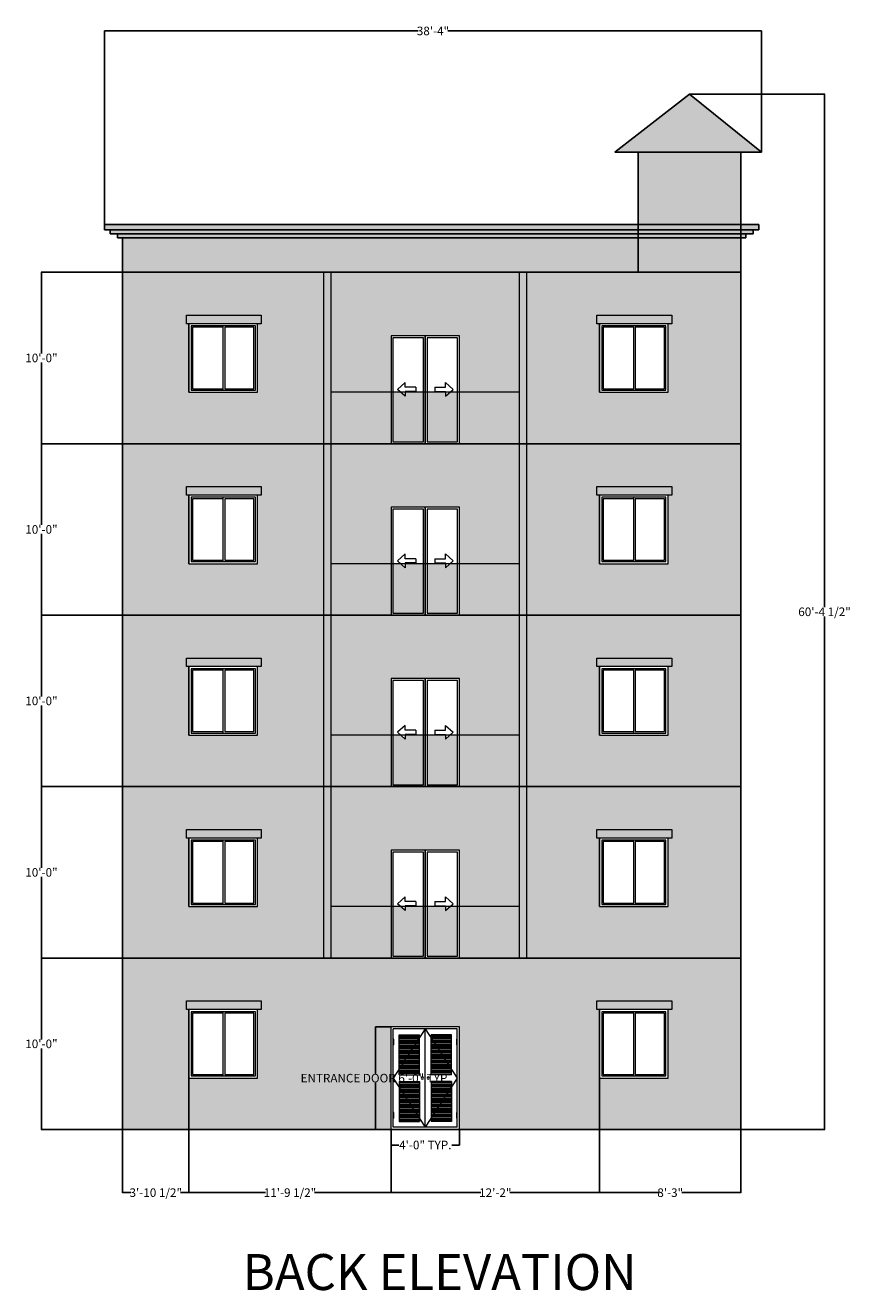
# Model space of a CAD drawing. Units: inches. Extents: x -113 to 5399, y -1393 to 3302.
# Tile 22 of 40: x 4822 to 5399, y -1393 to -507. Entities that reach past the tile are written whole.
import ezdxf

# ---------------------------------------------------------------- set-up
doc = ezdxf.new("R2010")
doc.units = ezdxf.units.IN
doc.header["$MEASUREMENT"] = 0
for name, color, linetype, lineweight in [('A-ANNO-DIMS', 254, 'Continuous', 18), ('A-ANNO-TEXT', 7, 'Continuous', 25), ('A-Door', 150, 'Continuous', 18), ('A-ELEV', 7, 'Continuous', 25), ('A-ELEV-GLAZ', 150, 'Continuous', 18), ('A-ELEV-RAIL', 7, 'Continuous', 18), ('A-ELEV-TRIM', 7, 'Continuous', 18), ('A-ELEV-TRIM-PATT', 7, 'Continuous', 13), ('A-ROOF', 7, 'Continuous', 25), ('A-ROOF-CORN-PATT', 3, 'Continuous', 13)]:
    doc.layers.add(name, color=color, linetype=linetype, lineweight=lineweight)
for name, color, linetype, lineweight, true_color in [('A-ELEV-RAIL-PATT', 9, 'Continuous', 13, 0xc7c8ca), ('A-ELEV-WALL-PATT', 241, 'Continuous', 13, 0xf7abae), ('A-ROOF-PATT', 251, 'Continuous', 13, 0x636466)]:
    doc.layers.add(name, color=color, linetype=linetype, lineweight=lineweight, true_color=true_color)
doc.styles.get("Standard").update_dxf_attribs({"font": 'arial.ttf'})
doc.dimstyles.get("Standard").update_dxf_attribs({"dimtxt": 6, "dimasz": 0.18, "dimexe": 0.18, "dimexo": 0.0625, "dimgap": 0.09, "dimtad": 0, "dimtih": 1, "dimtoh": 1, "dimdec": 1, "dimzin": 0, "dimdsep": 46, "dimlunit": 4, "dimtxsty": 'Standard', "dimblk": 'ARCHTICK', "dimcen": 0.09, "dimadec": 0, "dimazin": 0, "dimtfac": 1, "dimtdec": 1, "dimtofl": 0, "dimtmove": 0, "dimatfit": 3, "dimfxl": 1, "dimtolj": 1, "dimtzin": 0, "dimarcsym": 0})

# ---------------------------------------------------------------- blocks, each defined once
blk = doc.blocks.new('AE0C11')
for p, q in [((0, 0), (0, 1800)), ((0, 1800), (1200, 1800)), ((1200, 0), (1200, 1800)), ((40, 40), (40, 1760)), ((40, 1760), (1160, 1760)), ((600, 1760), (40, 900)), ((40, 1580), (50, 1580)), ((50, 1480), (50, 1580)), ((140, 1660), (500, 1660)), ((140, 960), (140, 1660)), ((140, 1635), (500, 1635)), ((140, 1610), (500, 1610)), ((140, 1585), (500, 1585)), ((140, 1560), (500, 1560)), ((500, 960), (500, 1660)), ((600, 40), (600, 1760)), ((600, 1760), (1160, 900)), ((700, 960), (700, 1660)), ((1060, 1660), (700, 1660)), ((1060, 1635), (700, 1635)), ((1060, 1610), (700, 1610)), ((1060, 1585), (700, 1585)), ((1060, 1560), (700, 1560)), ((1060, 960), (1060, 1660)), ((1150, 1480), (1150, 1580)), ((1150, 1580), (1160, 1580)), ((1160, 40), (1160, 1760)), ((40, 1480), (50, 1480)), ((140, 1535), (500, 1535)), ((140, 1510), (500, 1510)), ((140, 1485), (500, 1485)), ((140, 1460), (500, 1460)), ((140, 1435), (500, 1435)), ((140, 1410), (500, 1410)), ((140, 1385), (500, 1385)), ((140, 1360), (500, 1360)), ((140, 1335), (500, 1335)), ((1060, 1535), (700, 1535)), ((1060, 1510), (700, 1510)), ((1060, 1485), (700, 1485)), ((1060, 1460), (700, 1460)), ((1060, 1435), (700, 1435)), ((1060, 1410), (700, 1410)), ((1060, 1385), (700, 1385)), ((1060, 1360), (700, 1360)), ((1060, 1335), (700, 1335)), ((1150, 1480), (1160, 1480)), ((140, 1310), (500, 1310)), ((140, 1285), (500, 1285)), ((140, 1260), (500, 1260)), ((140, 1235), (500, 1235)), ((140, 1210), (500, 1210)), ((140, 1185), (500, 1185)), ((140, 1160), (500, 1160)), ((140, 1135), (500, 1135)), ((140, 1110), (500, 1110)), ((1060, 1310), (700, 1310)), ((1060, 1285), (700, 1285)), ((1060, 1260), (700, 1260)), ((1060, 1235), (700, 1235)), ((1060, 1210), (700, 1210)), ((1060, 1185), (700, 1185)), ((1060, 1160), (700, 1160)), ((1060, 1135), (700, 1135)), ((1060, 1110), (700, 1110)), ((40, 900), (600, 40)), ((140, 1085), (500, 1085)), ((140, 1060), (500, 1060)), ((140, 1035), (500, 1035)), ((140, 1010), (500, 1010)), ((140, 985), (500, 985)), ((140, 960), (500, 960)), ((1160, 900), (600, 40)), ((1060, 1085), (700, 1085)), ((1060, 1060), (700, 1060)), ((1060, 1035), (700, 1035)), ((1060, 1010), (700, 1010)), ((1060, 985), (700, 985)), ((1060, 960), (700, 960)), ((140, 840), (500, 840)), ((140, 840), (140, 140)), ((140, 815), (500, 815)), ((140, 790), (500, 790)), ((140, 765), (500, 765)), ((140, 740), (500, 740)), ((140, 715), (500, 715)), ((140, 690), (500, 690)), ((140, 665), (500, 665)), ((500, 840), (500, 140)), ((700, 840), (700, 140)), ((1060, 840), (700, 840)), ((1060, 815), (700, 815)), ((1060, 790), (700, 790)), ((1060, 765), (700, 765)), ((1060, 740), (700, 740)), ((1060, 715), (700, 715)), ((1060, 690), (700, 690)), ((1060, 665), (700, 665)), ((1060, 840), (1060, 140)), ((140, 640), (500, 640)), ((140, 615), (500, 615)), ((140, 590), (500, 590)), ((140, 565), (500, 565)), ((140, 540), (500, 540)), ((140, 515), (500, 515)), ((140, 490), (500, 490)), ((140, 465), (500, 465)), ((1060, 640), (700, 640)), ((1060, 615), (700, 615)), ((1060, 590), (700, 590)), ((1060, 565), (700, 565)), ((1060, 540), (700, 540)), ((1060, 515), (700, 515)), ((1060, 490), (700, 490)), ((1060, 465), (700, 465)), ((50, 300), (40, 300)), ((50, 200), (50, 300)), ((140, 440), (500, 440)), ((140, 415), (500, 415)), ((140, 390), (500, 390)), ((140, 365), (500, 365)), ((140, 340), (500, 340)), ((140, 315), (500, 315)), ((140, 290), (500, 290)), ((140, 265), (500, 265)), ((140, 240), (500, 240)), ((1060, 440), (700, 440)), ((1060, 415), (700, 415)), ((1060, 390), (700, 390)), ((1060, 365), (700, 365)), ((1060, 340), (700, 340)), ((1060, 315), (700, 315)), ((1060, 290), (700, 290)), ((1060, 265), (700, 265)), ((1060, 240), (700, 240)), ((1150, 300), (1160, 300)), ((1150, 200), (1150, 300)), ((0, 0), (1200, 0)), ((50, 200), (40, 200)), ((40, 40), (1160, 40)), ((140, 215), (500, 215)), ((140, 190), (500, 190)), ((140, 165), (500, 165)), ((140, 140), (500, 140)), ((1060, 215), (700, 215)), ((1060, 190), (700, 190)), ((1060, 165), (700, 165)), ((1060, 140), (700, 140)), ((1150, 200), (1160, 200))]:
    blk.add_line(p, q)
for centre in [(550, 900), (650, 900)]:
    blk.add_circle(centre, 20)
blk = doc.blocks.new('*U84')
for p, q in [((1.5, 1.5), (1.5, 46.5)), ((1.5, 46.5), (24, 46.5)), ((24, 1.5), (24, 46.5)), ((24, 46.5), (46.5, 46.5)), ((46.5, 46.5), (46.5, 1.5)), ((24, 1.5), (1.5, 1.5)), ((46.5, 1.5), (24, 1.5))]:
    blk.add_line(p, q)
blk.add_lwpolyline([(0, 0), (0, 48), (48, 48), (48, 0)], close=True)
for points in [[(23, 45.5), (23, 2.5), (2.5, 2.5), (2.5, 45.5), (23, 45.5)], [(24, 45.5), (45.5, 45.5), (45.5, 2.5), (24, 2.5)]]:
    blk.add_lwpolyline(points)
blk = doc.blocks.new('DOOR-SLIDING-PAIR-ELEV')
for p, q in [((9.94, 42.86), (4.53, 38.04)), ((9.94, 33.21), (4.53, 38.04)), ((9.94, 39.54), (9.94, 42.86)), ((17.43, 39.54), (9.94, 39.54)), ((17.43, 36.54), (9.94, 36.54)), ((9.94, 36.54), (9.94, 33.21)), ((17.43, 39.54), (17.43, 36.54)), ((30.57, 39.54), (38.06, 39.54)), ((30.57, 39.54), (30.57, 36.54)), ((30.57, 36.54), (38.06, 36.54)), ((38.06, 39.54), (38.06, 42.86)), ((38.06, 42.86), (43.47, 38.04)), ((38.06, 33.21), (43.47, 38.04)), ((38.06, 36.54), (38.06, 33.21))]:
    blk.add_line(p, q)
for points in [[(0, 75.57), (24, 75.57), (24, 0), (0, 0)], [(1.37, 74.2), (22.63, 74.2), (22.63, 1.37), (1.37, 1.37)], [(24, 75.57), (48, 75.57), (48, 0), (24, 0)], [(25.37, 74.2), (46.63, 74.2), (46.63, 1.37), (25.37, 1.37)]]:
    blk.add_lwpolyline(points, close=True)
blk = doc.blocks.new('_ArchTick')
at = {"color": 0, "linetype": 'ByBlock', "const_width": 0.15}
blk.add_lwpolyline([(-0.5, -0.5), (0.5, 0.5)], dxfattribs=at)
blk = doc.blocks.new('*D191')
at = {"layer": 'A-ANNO-DIMS', "color": 0, "lineweight": -2, "transparency": 16777216}
for p, q in [((5078.07, -1208.13), (5067.16, -1208.13)), ((5067.34, -1208.13), (5067.34, -1240.94)), ((5067.34, -1280.13), (5067.34, -1247.33)), ((5078.07, -1280.13), (5067.16, -1280.13))]:
    blk.add_line(p, q, dxfattribs=at)
at = {"layer": 'Defpoints', "color": 0, "transparency": 16777216}
for p in [(5067.34, -1208.13), (5078.14, -1208.13), (5078.14, -1280.13)]:
    blk.add_point(p, dxfattribs=at)
at = {"layer": 'A-ANNO-DIMS', "color": 0, "lineweight": -2, "transparency": 16777216, "xscale": 0.18, "yscale": 0.18, "zscale": 0.18}
for p, rotation in [((5067.34, -1208.13), 90), ((5067.34, -1280.13), 270)]:
    blk.add_blockref('_ArchTick', p, dxfattribs=dict(at, rotation=rotation))
at = {"layer": 'A-ANNO-DIMS', "color": 0, "transparency": 16777216, "insert": (5067.34, -1244.13), "char_height": 6, "attachment_point": 5}
blk.add_mtext('\\A1;ENTRANCE DOOR 6\'-0" TYP.', dxfattribs=at)
blk = doc.blocks.new('*D192')
at = {"layer": 'A-ANNO-DIMS', "color": 0, "lineweight": -2, "transparency": 16777216}
for p, q in [((5078.14, -1280.2), (5078.14, -1291.11)), ((5126.14, -1280.2), (5126.14, -1291.11)), ((5078.14, -1290.93), (5083.64, -1290.93)), ((5126.14, -1290.93), (5120.63, -1290.93))]:
    blk.add_line(p, q, dxfattribs=at)
at = {"layer": 'Defpoints', "color": 0, "transparency": 16777216}
for p in [(5078.14, -1280.13), (5126.14, -1280.13), (5078.14, -1290.93)]:
    blk.add_point(p, dxfattribs=at)
at = {"layer": 'A-ANNO-DIMS', "color": 0, "lineweight": -2, "transparency": 16777216, "xscale": 0.18, "yscale": 0.18, "zscale": 0.18, "rotation": 180}
blk.add_blockref('_ArchTick', (5078.14, -1290.93), dxfattribs=at)
at = {"layer": 'A-ANNO-DIMS', "color": 0, "lineweight": -2, "transparency": 16777216, "xscale": 0.18, "yscale": 0.18, "zscale": 0.18}
blk.add_blockref('_ArchTick', (5126.14, -1290.93), dxfattribs=at)
at = {"layer": 'A-ANNO-DIMS', "color": 0, "transparency": 16777216, "insert": (5102.14, -1290.93), "char_height": 6, "attachment_point": 5}
blk.add_mtext('\\A1;4\'-0" TYP.', dxfattribs=at)
blk = doc.blocks.new('*D229')
at = {"layer": 'A-ANNO-DIMS', "color": 0, "lineweight": -2, "transparency": 16777216}
for p, q in [((4877.49, -646.59), (4877.49, -511.08)), ((4877.49, -511.26), (5097.12, -511.26)), ((5337.54, -511.26), (5117.91, -511.26)), ((5337.54, -596.07), (5337.54, -511.08))]:
    blk.add_line(p, q, dxfattribs=at)
at = {"layer": 'Defpoints', "color": 0, "transparency": 16777216}
for p in [(5337.54, -511.26), (5337.54, -596.13), (4877.49, -646.65)]:
    blk.add_point(p, dxfattribs=at)
at = {"layer": 'A-ANNO-DIMS', "color": 0, "lineweight": -2, "transparency": 16777216, "xscale": 0.18, "yscale": 0.18, "zscale": 0.18, "rotation": 180}
blk.add_blockref('_ArchTick', (4877.49, -511.26), dxfattribs=at)
at = {"layer": 'A-ANNO-DIMS', "color": 0, "lineweight": -2, "transparency": 16777216, "xscale": 0.18, "yscale": 0.18, "zscale": 0.18}
blk.add_blockref('_ArchTick', (5337.54, -511.26), dxfattribs=at)
at = {"layer": 'A-ANNO-DIMS', "color": 0, "transparency": 16777216, "insert": (5107.51, -511.26), "char_height": 6, "attachment_point": 5}
blk.add_mtext('\\A1;38\'-4"', dxfattribs=at)
blk = doc.blocks.new('*D230')
at = {"layer": 'A-ANNO-DIMS', "color": 0, "lineweight": -2, "transparency": 16777216}
for p, q in [((5287.2, -555.41), (5381.87, -555.41)), ((5381.69, -555.41), (5381.69, -914.58)), ((5381.69, -1280.13), (5381.69, -920.96)), ((5323.2, -1280.13), (5381.87, -1280.13))]:
    blk.add_line(p, q, dxfattribs=at)
at = {"layer": 'Defpoints', "color": 0, "transparency": 16777216}
for p in [(5287.14, -555.41), (5381.69, -555.41), (5323.14, -1280.13)]:
    blk.add_point(p, dxfattribs=at)
at = {"layer": 'A-ANNO-DIMS', "color": 0, "lineweight": -2, "transparency": 16777216, "xscale": 0.18, "yscale": 0.18, "zscale": 0.18}
for p, rotation in [((5381.69, -555.41), 90), ((5381.69, -1280.13), 270)]:
    blk.add_blockref('_ArchTick', p, dxfattribs=dict(at, rotation=rotation))
at = {"layer": 'A-ANNO-DIMS', "color": 0, "transparency": 16777216, "insert": (5381.69, -917.77), "char_height": 6, "attachment_point": 5}
blk.add_mtext('\\A1;60\'-4 1/2"', dxfattribs=at)
blk = doc.blocks.new('*D231')
at = {"layer": 'A-ANNO-DIMS', "color": 0, "lineweight": -2, "transparency": 16777216}
for p, q in [((4890.07, -1160.13), (4833.16, -1160.13)), ((4833.34, -1160.13), (4833.34, -1216.98)), ((4833.34, -1280.13), (4833.34, -1223.29)), ((4890.07, -1280.13), (4833.16, -1280.13))]:
    blk.add_line(p, q, dxfattribs=at)
at = {"layer": 'Defpoints', "color": 0, "transparency": 16777216}
for p in [(4833.34, -1160.13), (4890.14, -1160.13), (4890.14, -1280.13)]:
    blk.add_point(p, dxfattribs=at)
at = {"layer": 'A-ANNO-DIMS', "color": 0, "lineweight": -2, "transparency": 16777216, "xscale": 0.18, "yscale": 0.18, "zscale": 0.18}
for p, rotation in [((4833.34, -1160.13), 90), ((4833.34, -1280.13), 270)]:
    blk.add_blockref('_ArchTick', p, dxfattribs=dict(at, rotation=rotation))
at = {"layer": 'A-ANNO-DIMS', "color": 0, "transparency": 16777216, "insert": (4833.34, -1220.13), "char_height": 6, "attachment_point": 5}
blk.add_mtext('\\A1;10\'-0"', dxfattribs=at)
blk = doc.blocks.new('*D232')
at = {"layer": 'A-ANNO-DIMS', "color": 0, "lineweight": -2, "transparency": 16777216}
for p, q in [((4890.07, -1040.13), (4833.16, -1040.13)), ((4833.34, -1040.13), (4833.34, -1096.98)), ((4833.34, -1160.13), (4833.34, -1103.29)), ((4890.07, -1160.13), (4833.16, -1160.13))]:
    blk.add_line(p, q, dxfattribs=at)
at = {"layer": 'Defpoints', "color": 0, "transparency": 16777216}
for p in [(4833.34, -1040.13), (4890.14, -1040.13), (4890.14, -1160.13)]:
    blk.add_point(p, dxfattribs=at)
at = {"layer": 'A-ANNO-DIMS', "color": 0, "lineweight": -2, "transparency": 16777216, "xscale": 0.18, "yscale": 0.18, "zscale": 0.18}
for p, rotation in [((4833.34, -1040.13), 90), ((4833.34, -1160.13), 270)]:
    blk.add_blockref('_ArchTick', p, dxfattribs=dict(at, rotation=rotation))
at = {"layer": 'A-ANNO-DIMS', "color": 0, "transparency": 16777216, "insert": (4833.34, -1100.13), "char_height": 6, "attachment_point": 5}
blk.add_mtext('\\A1;10\'-0"', dxfattribs=at)
blk = doc.blocks.new('*D233')
at = {"layer": 'A-ANNO-DIMS', "color": 0, "lineweight": -2, "transparency": 16777216}
for p, q in [((4890.07, -920.13), (4833.16, -920.13)), ((4833.34, -920.13), (4833.34, -976.98)), ((4833.34, -1040.13), (4833.34, -983.29)), ((4890.07, -1040.13), (4833.16, -1040.13))]:
    blk.add_line(p, q, dxfattribs=at)
at = {"layer": 'Defpoints', "color": 0, "transparency": 16777216}
for p in [(4833.34, -920.13), (4890.14, -920.13), (4890.14, -1040.13)]:
    blk.add_point(p, dxfattribs=at)
at = {"layer": 'A-ANNO-DIMS', "color": 0, "lineweight": -2, "transparency": 16777216, "xscale": 0.18, "yscale": 0.18, "zscale": 0.18}
for p, rotation in [((4833.34, -920.13), 90), ((4833.34, -1040.13), 270)]:
    blk.add_blockref('_ArchTick', p, dxfattribs=dict(at, rotation=rotation))
at = {"layer": 'A-ANNO-DIMS', "color": 0, "transparency": 16777216, "insert": (4833.34, -980.13), "char_height": 6, "attachment_point": 5}
blk.add_mtext('\\A1;10\'-0"', dxfattribs=at)
blk = doc.blocks.new('*D234')
at = {"layer": 'A-ANNO-DIMS', "color": 0, "lineweight": -2, "transparency": 16777216}
for p, q in [((4890.07, -800.13), (4833.16, -800.13)), ((4833.34, -800.13), (4833.34, -856.98)), ((4833.34, -920.13), (4833.34, -863.29)), ((4890.07, -920.13), (4833.16, -920.13))]:
    blk.add_line(p, q, dxfattribs=at)
at = {"layer": 'Defpoints', "color": 0, "transparency": 16777216}
for p in [(4833.34, -800.13), (4890.14, -800.13), (4890.14, -920.13)]:
    blk.add_point(p, dxfattribs=at)
at = {"layer": 'A-ANNO-DIMS', "color": 0, "lineweight": -2, "transparency": 16777216, "xscale": 0.18, "yscale": 0.18, "zscale": 0.18}
for p, rotation in [((4833.34, -800.13), 90), ((4833.34, -920.13), 270)]:
    blk.add_blockref('_ArchTick', p, dxfattribs=dict(at, rotation=rotation))
at = {"layer": 'A-ANNO-DIMS', "color": 0, "transparency": 16777216, "insert": (4833.34, -860.13), "char_height": 6, "attachment_point": 5}
blk.add_mtext('\\A1;10\'-0"', dxfattribs=at)
blk = doc.blocks.new('*D235')
at = {"layer": 'A-ANNO-DIMS', "color": 0, "lineweight": -2, "transparency": 16777216}
for p, q in [((4890.07, -680.13), (4833.16, -680.13)), ((4833.34, -680.13), (4833.34, -736.98)), ((4833.34, -800.13), (4833.34, -743.29)), ((4890.07, -800.13), (4833.16, -800.13))]:
    blk.add_line(p, q, dxfattribs=at)
at = {"layer": 'Defpoints', "color": 0, "transparency": 16777216}
for p in [(4833.34, -680.13), (4890.14, -680.13), (4890.14, -800.13)]:
    blk.add_point(p, dxfattribs=at)
at = {"layer": 'A-ANNO-DIMS', "color": 0, "lineweight": -2, "transparency": 16777216, "xscale": 0.18, "yscale": 0.18, "zscale": 0.18}
for p, rotation in [((4833.34, -680.13), 90), ((4833.34, -800.13), 270)]:
    blk.add_blockref('_ArchTick', p, dxfattribs=dict(at, rotation=rotation))
at = {"layer": 'A-ANNO-DIMS', "color": 0, "transparency": 16777216, "insert": (4833.34, -740.13), "char_height": 6, "attachment_point": 5}
blk.add_mtext('\\A1;10\'-0"', dxfattribs=at)
blk = doc.blocks.new('*D236')
at = {"layer": 'A-ANNO-DIMS', "color": 0, "lineweight": -2, "transparency": 16777216}
for p, q in [((4936.64, -1244.2), (4936.64, -1324.46)), ((4890.14, -1280.2), (4890.14, -1324.46)), ((4890.14, -1324.28), (4896, -1324.28)), ((4936.64, -1324.28), (4930.77, -1324.28))]:
    blk.add_line(p, q, dxfattribs=at)
at = {"layer": 'Defpoints', "color": 0, "transparency": 16777216}
for p in [(4936.64, -1244.13), (4890.14, -1280.13), (4936.64, -1324.28)]:
    blk.add_point(p, dxfattribs=at)
at = {"layer": 'A-ANNO-DIMS', "color": 0, "lineweight": -2, "transparency": 16777216, "xscale": 0.18, "yscale": 0.18, "zscale": 0.18, "rotation": 180}
blk.add_blockref('_ArchTick', (4890.14, -1324.28), dxfattribs=at)
at = {"layer": 'A-ANNO-DIMS', "color": 0, "lineweight": -2, "transparency": 16777216, "xscale": 0.18, "yscale": 0.18, "zscale": 0.18}
blk.add_blockref('_ArchTick', (4936.64, -1324.28), dxfattribs=at)
at = {"layer": 'A-ANNO-DIMS', "color": 0, "transparency": 16777216, "insert": (4913.39, -1324.28), "char_height": 6, "attachment_point": 5}
blk.add_mtext('\\A1;3\'-10 1/2"', dxfattribs=at)
blk = doc.blocks.new('*D237')
at = {"layer": 'A-ANNO-DIMS', "color": 0, "lineweight": -2, "transparency": 16777216}
for p, q in [((4936.64, -1244.2), (4936.64, -1324.46)), ((5078.14, -1280.2), (5078.14, -1324.46)), ((4936.64, -1324.28), (4990.28, -1324.28)), ((5078.14, -1324.28), (5024.49, -1324.28))]:
    blk.add_line(p, q, dxfattribs=at)
at = {"layer": 'Defpoints', "color": 0, "transparency": 16777216}
for p in [(4936.64, -1244.13), (5078.14, -1280.13), (5078.14, -1324.28)]:
    blk.add_point(p, dxfattribs=at)
at = {"layer": 'A-ANNO-DIMS', "color": 0, "lineweight": -2, "transparency": 16777216, "xscale": 0.18, "yscale": 0.18, "zscale": 0.18, "rotation": 180}
blk.add_blockref('_ArchTick', (4936.64, -1324.28), dxfattribs=at)
at = {"layer": 'A-ANNO-DIMS', "color": 0, "lineweight": -2, "transparency": 16777216, "xscale": 0.18, "yscale": 0.18, "zscale": 0.18}
blk.add_blockref('_ArchTick', (5078.14, -1324.28), dxfattribs=at)
at = {"layer": 'A-ANNO-DIMS', "color": 0, "transparency": 16777216, "insert": (5007.39, -1324.28), "char_height": 6, "attachment_point": 5}
blk.add_mtext('\\A1;11\'-9 1/2"', dxfattribs=at)
blk = doc.blocks.new('*D238')
at = {"layer": 'A-ANNO-DIMS', "color": 0, "lineweight": -2, "transparency": 16777216}
for p, q in [((5224.14, -1244.2), (5224.14, -1324.46)), ((5078.14, -1280.2), (5078.14, -1324.46)), ((5078.14, -1324.28), (5141.02, -1324.28)), ((5224.14, -1324.28), (5161.25, -1324.28))]:
    blk.add_line(p, q, dxfattribs=at)
at = {"layer": 'Defpoints', "color": 0, "transparency": 16777216}
for p in [(5224.14, -1244.13), (5078.14, -1280.13), (5224.14, -1324.28)]:
    blk.add_point(p, dxfattribs=at)
at = {"layer": 'A-ANNO-DIMS', "color": 0, "lineweight": -2, "transparency": 16777216, "xscale": 0.18, "yscale": 0.18, "zscale": 0.18, "rotation": 180}
blk.add_blockref('_ArchTick', (5078.14, -1324.28), dxfattribs=at)
at = {"layer": 'A-ANNO-DIMS', "color": 0, "lineweight": -2, "transparency": 16777216, "xscale": 0.18, "yscale": 0.18, "zscale": 0.18}
blk.add_blockref('_ArchTick', (5224.14, -1324.28), dxfattribs=at)
at = {"layer": 'A-ANNO-DIMS', "color": 0, "transparency": 16777216, "insert": (5151.14, -1324.28), "char_height": 6, "attachment_point": 5}
blk.add_mtext('\\A1;12\'-2"', dxfattribs=at)
blk = doc.blocks.new('*D239')
at = {"layer": 'A-ANNO-DIMS', "color": 0, "lineweight": -2, "transparency": 16777216}
for p, q in [((5224.14, -1244.2), (5224.14, -1324.46)), ((5323.14, -1280.2), (5323.14, -1324.46)), ((5224.14, -1324.28), (5265.57, -1324.28)), ((5323.14, -1324.28), (5281.71, -1324.28))]:
    blk.add_line(p, q, dxfattribs=at)
at = {"layer": 'Defpoints', "color": 0, "transparency": 16777216}
for p in [(5224.14, -1244.13), (5323.14, -1280.13), (5323.14, -1324.28)]:
    blk.add_point(p, dxfattribs=at)
at = {"layer": 'A-ANNO-DIMS', "color": 0, "lineweight": -2, "transparency": 16777216, "xscale": 0.18, "yscale": 0.18, "zscale": 0.18, "rotation": 180}
blk.add_blockref('_ArchTick', (5224.14, -1324.28), dxfattribs=at)
at = {"layer": 'A-ANNO-DIMS', "color": 0, "lineweight": -2, "transparency": 16777216, "xscale": 0.18, "yscale": 0.18, "zscale": 0.18}
blk.add_blockref('_ArchTick', (5323.14, -1324.28), dxfattribs=at)
at = {"layer": 'A-ANNO-DIMS', "color": 0, "transparency": 16777216, "insert": (5273.64, -1324.28), "char_height": 6, "attachment_point": 5}
blk.add_mtext('\\A1;8\'-3"', dxfattribs=at)

msp = doc.modelspace()

# ---------------------------------------------------------------- hatches: boundary and pattern name
at = {"layer": 'A-ELEV-RAIL-PATT', "transparency": 33554498}
h = msp.add_hatch(color=256, dxfattribs=at)
h.dxf.hatch_style = 1
h.paths.add_polyline_path([(5126.14, -764.13), (5168.14, -764.13), (5168.14, -800.13), (5126.14, -800.13)])
h.paths.add_polyline_path([(5036.14, -764.13), (5078.14, -764.13), (5078.14, -800.13), (5036.14, -800.13)])
h.paths.add_polyline_path([(5079.51, -764.13), (5084.95, -764.13), (5088.08, -766.92), (5088.08, -764.13), (5100.77, -764.13), (5100.77, -798.76), (5079.51, -798.76)])
h.paths.add_polyline_path([(5103.51, -764.13), (5116.2, -764.13), (5116.2, -766.92), (5119.32, -764.13), (5124.77, -764.13), (5124.77, -798.76), (5103.51, -798.76)])
h = msp.add_hatch(color=256, dxfattribs=at)
h.dxf.hatch_style = 1
h.paths.add_polyline_path([(5126.14, -884.13), (5168.14, -884.13), (5168.14, -920.13), (5126.14, -920.13)])
h.paths.add_polyline_path([(5036.14, -884.13), (5078.14, -884.13), (5078.14, -920.13), (5036.14, -920.13)])
h.paths.add_polyline_path([(5079.51, -884.13), (5084.95, -884.13), (5088.08, -886.92), (5088.08, -884.13), (5100.77, -884.13), (5100.77, -918.76), (5079.51, -918.76)])
h.paths.add_polyline_path([(5103.51, -884.13), (5116.2, -884.13), (5116.2, -886.92), (5119.32, -884.13), (5124.77, -884.13), (5124.77, -918.76), (5103.51, -918.76)])
h = msp.add_hatch(color=256, dxfattribs=at)
h.dxf.hatch_style = 1
h.paths.add_polyline_path([(5126.14, -1004.13), (5168.14, -1004.13), (5168.14, -1040.13), (5126.14, -1040.13)])
h.paths.add_polyline_path([(5036.14, -1004.13), (5078.14, -1004.13), (5078.14, -1040.13), (5036.14, -1040.13)])
h.paths.add_polyline_path([(5079.51, -1004.13), (5084.95, -1004.13), (5088.08, -1006.92), (5088.08, -1004.13), (5100.77, -1004.13), (5100.77, -1038.76), (5079.51, -1038.76)])
h.paths.add_polyline_path([(5103.51, -1004.13), (5116.2, -1004.13), (5116.2, -1006.92), (5119.32, -1004.13), (5124.77, -1004.13), (5124.77, -1038.76), (5103.51, -1038.76)])
h = msp.add_hatch(color=256, dxfattribs=at)
h.dxf.hatch_style = 1
h.paths.add_polyline_path([(5126.14, -1124.13), (5168.14, -1124.13), (5168.14, -1160.13), (5126.14, -1160.13)])
h.paths.add_polyline_path([(5036.14, -1124.13), (5078.14, -1124.13), (5078.14, -1160.13), (5036.14, -1160.13)])
h.paths.add_polyline_path([(5079.51, -1124.13), (5084.95, -1124.13), (5088.08, -1126.92), (5088.08, -1124.13), (5100.77, -1124.13), (5100.77, -1158.76), (5079.51, -1158.76)])
h.paths.add_polyline_path([(5103.51, -1124.13), (5116.2, -1124.13), (5116.2, -1126.92), (5119.32, -1124.13), (5124.77, -1124.13), (5124.77, -1158.76), (5103.51, -1158.76)])
at = {"layer": 'A-ELEV-TRIM-PATT'}
h = msp.add_hatch(color=256, dxfattribs=at)
h.dxf.hatch_style = 1
h.paths.add_polyline_path([(4890.14, -656.13), (5323.14, -656.13), (5323.14, -680.13), (4890.14, -680.13)])
h = msp.add_hatch(color=256, dxfattribs=at)
h.dxf.hatch_style = 1
h.paths.add_polyline_path([(5031.14, -1040.13), (5036.14, -1040.13), (5036.14, -1160.13), (5031.14, -1160.13)])
h.paths.add_polyline_path([(5031.14, -920.13), (5036.14, -920.13), (5036.14, -1040.13), (5031.14, -1040.13)])
h.paths.add_polyline_path([(5031.14, -800.13), (5036.14, -800.13), (5036.14, -920.13), (5031.14, -920.13)])
h.paths.add_polyline_path([(5031.14, -680.13), (5036.14, -680.13), (5036.14, -800.13), (5031.14, -800.13)])
h.paths.add_polyline_path([(5168.14, -680.13), (5173.14, -680.13), (5173.14, -800.13), (5168.14, -800.13)])
h.paths.add_polyline_path([(5168.14, -800.13), (5173.14, -800.13), (5173.14, -920.13), (5168.14, -920.13)])
h.paths.add_polyline_path([(5168.14, -920.13), (5173.14, -920.13), (5173.14, -1040.13), (5168.14, -1040.13)])
h.paths.add_polyline_path([(5168.14, -1040.13), (5173.14, -1040.13), (5173.14, -1160.13), (5168.14, -1160.13)])
h = msp.add_hatch(color=256, dxfattribs=at)
h.dxf.hatch_style = 1
h.paths.add_polyline_path([(4934.82, -1190.14), (4987.23, -1190.14), (4987.23, -1196.13), (4934.82, -1196.13)])
h.paths.add_polyline_path([(5222.32, -1190.14), (5274.73, -1190.14), (5274.73, -1196.13), (5222.32, -1196.13)])
h.paths.add_polyline_path([(5222.32, -1070.14), (5274.73, -1070.14), (5274.73, -1076.13), (5222.32, -1076.13)])
h.paths.add_polyline_path([(5222.32, -950.14), (5274.73, -950.14), (5274.73, -956.13), (5222.32, -956.13)])
h.paths.add_polyline_path([(5222.32, -830.14), (5274.73, -830.14), (5274.73, -836.13), (5222.32, -836.13)])
h.paths.add_polyline_path([(4934.82, -830.14), (4987.23, -830.14), (4987.23, -836.13), (4934.82, -836.13)])
h.paths.add_polyline_path([(4934.82, -710.14), (4987.23, -710.14), (4987.23, -716.13), (4934.82, -716.13)])
h.paths.add_polyline_path([(5222.32, -710.14), (5274.73, -710.14), (5274.73, -716.13), (5222.32, -716.13)])
h.paths.add_polyline_path([(4934.82, -1070.14), (4987.23, -1070.14), (4987.23, -1076.13), (4934.82, -1076.13)])
h.paths.add_polyline_path([(4934.82, -950.14), (4987.23, -950.14), (4987.23, -956.13), (4934.82, -956.13)])
at = {"layer": 'A-ELEV-WALL-PATT'}
h = msp.add_hatch(color=256, dxfattribs=at)
h.dxf.hatch_style = 1
h.paths.add_polyline_path([(5251.14, -596.13), (5323.14, -596.13), (5323.14, -680.13), (5251.14, -680.13)])
h = msp.add_hatch(color=256, dxfattribs=at)
h.dxf.hatch_style = 1
h.paths.add_polyline_path([(5173.14, -680.13), (5323.14, -680.13), (5323.14, -800.13), (5173.14, -800.13)])
h.paths.add_polyline_path([(5222.32, -716.13), (5224.14, -716.13), (5224.14, -764.13), (5272.14, -764.13), (5272.14, -716.13), (5274.73, -716.13), (5274.73, -710.14), (5222.32, -710.14)], flags=16)
h.paths.add_polyline_path([(5225.64, -717.63), (5225.64, -762.63), (5248.14, -762.63), (5270.64, -762.63), (5270.64, -717.63), (5248.14, -717.63)], flags=0)
h.paths.add_polyline_path([(5226.64, -718.63), (5226.64, -761.63), (5248.14, -761.63), (5248.14, -718.63)], flags=0)
h.paths.add_polyline_path([(5249.14, -761.63), (5269.64, -761.63), (5269.64, -718.63), (5249.14, -718.63)], flags=0)
h.paths.add_polyline_path([(5036.14, -680.13), (5168.14, -680.13), (5168.14, -764.13), (5126.14, -764.13), (5126.14, -724.56), (5102.14, -724.56), (5078.14, -724.56), (5078.14, -764.13), (5036.14, -764.13)])
h.paths.add_polyline_path([(4890.14, -680.13), (5031.14, -680.13), (5031.14, -800.13), (4890.14, -800.13)])
h.paths.add_polyline_path([(4984.64, -716.13), (4987.23, -716.13), (4987.23, -710.14), (4934.82, -710.14), (4934.82, -716.13), (4936.64, -716.13), (4936.64, -764.13), (4984.64, -764.13)], flags=16)
h.paths.add_polyline_path([(4983.14, -717.63), (4960.64, -717.63), (4938.14, -717.63), (4938.14, -762.63), (4960.64, -762.63), (4983.14, -762.63)], flags=0)
h.paths.add_polyline_path([(4982.14, -718.63), (4961.64, -718.63), (4961.64, -761.63), (4982.14, -761.63)], flags=0)
h.paths.add_polyline_path([(4960.64, -718.63), (4939.14, -718.63), (4939.14, -761.63), (4960.64, -761.63)], flags=0)
h.paths.add_polyline_path([(4890.14, -800.13), (5031.14, -800.13), (5031.14, -920.13), (4890.14, -920.13)])
h.paths.add_polyline_path([(4987.23, -836.13), (4987.23, -830.14), (4934.82, -830.14), (4934.82, -836.13), (4936.64, -836.13), (4936.64, -884.13), (4984.64, -884.13), (4984.64, -836.13)], flags=16)
h.paths.add_polyline_path([(4983.14, -837.63), (4960.64, -837.63), (4938.14, -837.63), (4938.14, -882.63), (4960.64, -882.63), (4983.14, -882.63)], flags=0)
h.paths.add_polyline_path([(4982.14, -838.63), (4961.64, -838.63), (4961.64, -881.63), (4982.14, -881.63)], flags=0)
h.paths.add_polyline_path([(4960.64, -838.63), (4939.14, -838.63), (4939.14, -881.63), (4960.64, -881.63)], flags=0)
h.paths.add_polyline_path([(5036.14, -800.13), (5168.14, -800.13), (5168.14, -884.13), (5126.14, -884.13), (5126.14, -844.56), (5102.14, -844.56), (5078.14, -844.56), (5078.14, -884.13), (5036.14, -884.13)])
h.paths.add_polyline_path([(5173.14, -800.13), (5323.14, -800.13), (5323.14, -920.13), (5173.14, -920.13)])
h.paths.add_polyline_path([(5224.14, -884.13), (5272.14, -884.13), (5272.14, -836.13), (5274.73, -836.13), (5274.73, -830.14), (5222.32, -830.14), (5222.32, -836.13), (5224.14, -836.13)], flags=16)
h.paths.add_polyline_path([(5225.64, -882.63), (5248.14, -882.63), (5270.64, -882.63), (5270.64, -837.63), (5248.14, -837.63), (5225.64, -837.63)], flags=0)
h.paths.add_polyline_path([(5226.64, -881.63), (5248.14, -881.63), (5248.14, -838.63), (5226.64, -838.63)], flags=0)
h.paths.add_polyline_path([(5249.14, -881.63), (5269.64, -881.63), (5269.64, -838.63), (5249.14, -838.63)], flags=0)
h.paths.add_polyline_path([(5173.14, -920.13), (5323.14, -920.13), (5323.14, -1040.13), (5173.14, -1040.13)])
h.paths.add_polyline_path([(5224.14, -1004.13), (5272.14, -1004.13), (5272.14, -956.13), (5274.73, -956.13), (5274.73, -950.14), (5222.32, -950.14), (5222.32, -956.13), (5224.14, -956.13)], flags=16)
h.paths.add_polyline_path([(5225.64, -1002.63), (5248.14, -1002.63), (5270.64, -1002.63), (5270.64, -957.63), (5248.14, -957.63), (5225.64, -957.63)], flags=0)
h.paths.add_polyline_path([(5226.64, -1001.63), (5248.14, -1001.63), (5248.14, -958.63), (5226.64, -958.63)], flags=0)
h.paths.add_polyline_path([(5249.14, -1001.63), (5269.64, -1001.63), (5269.64, -958.63), (5249.14, -958.63)], flags=0)
h.paths.add_polyline_path([(5036.14, -920.13), (5168.14, -920.13), (5168.14, -1004.13), (5126.14, -1004.13), (5126.14, -964.56), (5102.14, -964.56), (5078.14, -964.56), (5078.14, -1004.13), (5036.14, -1004.13)])
h.paths.add_polyline_path([(4890.14, -920.13), (5031.14, -920.13), (5031.14, -1040.13), (4890.14, -1040.13)])
h.paths.add_polyline_path([(4984.64, -956.13), (4987.23, -956.13), (4987.23, -950.14), (4934.82, -950.14), (4934.82, -956.13), (4936.64, -956.13), (4936.64, -1004.13), (4984.64, -1004.13)], flags=16)
h.paths.add_polyline_path([(4983.14, -957.63), (4960.64, -957.63), (4938.14, -957.63), (4938.14, -1002.63), (4960.64, -1002.63), (4983.14, -1002.63)], flags=0)
h.paths.add_polyline_path([(4982.14, -958.63), (4961.64, -958.63), (4961.64, -1001.63), (4982.14, -1001.63)], flags=0)
h.paths.add_polyline_path([(4960.64, -958.63), (4939.14, -958.63), (4939.14, -1001.63), (4960.64, -1001.63)], flags=0)
h.paths.add_polyline_path([(4890.14, -1040.13), (5031.14, -1040.13), (5031.14, -1160.13), (4890.14, -1160.13)])
h.paths.add_polyline_path([(4984.64, -1076.13), (4987.23, -1076.13), (4987.23, -1070.14), (4934.82, -1070.14), (4934.82, -1076.13), (4936.64, -1076.13), (4936.64, -1124.13), (4984.64, -1124.13)], flags=16)
h.paths.add_polyline_path([(4983.14, -1077.63), (4960.64, -1077.63), (4938.14, -1077.63), (4938.14, -1122.63), (4960.64, -1122.63), (4983.14, -1122.63)], flags=0)
h.paths.add_polyline_path([(4982.14, -1078.63), (4961.64, -1078.63), (4961.64, -1121.63), (4982.14, -1121.63)], flags=0)
h.paths.add_polyline_path([(4960.64, -1078.63), (4939.14, -1078.63), (4939.14, -1121.63), (4960.64, -1121.63)], flags=0)
h.paths.add_polyline_path([(5036.14, -1040.13), (5168.14, -1040.13), (5168.14, -1124.13), (5126.14, -1124.13), (5126.14, -1084.56), (5102.14, -1084.56), (5078.14, -1084.56), (5078.14, -1124.13), (5036.14, -1124.13)])
h.paths.add_polyline_path([(5173.14, -1040.13), (5323.14, -1040.13), (5323.14, -1160.13), (5173.14, -1160.13)])
h.paths.add_polyline_path([(5224.14, -1124.13), (5272.14, -1124.13), (5272.14, -1076.13), (5274.73, -1076.13), (5274.73, -1070.14), (5222.32, -1070.14), (5222.32, -1076.13), (5224.14, -1076.13)], flags=16)
h.paths.add_polyline_path([(5225.64, -1122.63), (5248.14, -1122.63), (5270.64, -1122.63), (5270.64, -1077.63), (5248.14, -1077.63), (5225.64, -1077.63)], flags=0)
h.paths.add_polyline_path([(5226.64, -1121.63), (5248.14, -1121.63), (5248.14, -1078.63), (5226.64, -1078.63)], flags=0)
h.paths.add_polyline_path([(5249.14, -1121.63), (5269.64, -1121.63), (5269.64, -1078.63), (5249.14, -1078.63)], flags=0)
h.paths.add_polyline_path([(5126.14, -1208.13), (5078.14, -1208.13), (5078.14, -1280.13), (4890.14, -1280.13), (4890.14, -1160.13), (5031.14, -1160.13), (5323.14, -1160.13), (5323.14, -1280.13), (5126.14, -1280.13)])
h.paths.add_polyline_path([(5224.14, -1244.13), (5272.14, -1244.13), (5272.14, -1196.13), (5274.73, -1196.13), (5274.73, -1190.14), (5222.32, -1190.14), (5222.32, -1196.13), (5224.14, -1196.13)], flags=16)
h.paths.add_polyline_path([(5225.64, -1242.63), (5248.14, -1242.63), (5270.64, -1242.63), (5270.64, -1197.63), (5248.14, -1197.63), (5225.64, -1197.63)], flags=0)
h.paths.add_polyline_path([(5226.64, -1241.63), (5248.14, -1241.63), (5248.14, -1198.63), (5226.64, -1198.63)], flags=0)
h.paths.add_polyline_path([(5249.14, -1241.63), (5269.64, -1241.63), (5269.64, -1198.63), (5249.14, -1198.63)], flags=0)
h.paths.add_polyline_path([(4987.23, -1196.13), (4987.23, -1190.14), (4934.82, -1190.14), (4934.82, -1196.13), (4936.64, -1196.13), (4936.64, -1244.13), (4984.64, -1244.13), (4984.64, -1196.13)], flags=16)
h.paths.add_polyline_path([(4983.14, -1197.63), (4960.64, -1197.63), (4938.14, -1197.63), (4938.14, -1242.63), (4960.64, -1242.63), (4983.14, -1242.63)], flags=0)
h.paths.add_polyline_path([(4982.14, -1198.63), (4961.64, -1198.63), (4961.64, -1241.63), (4982.14, -1241.63)], flags=0)
h.paths.add_polyline_path([(4960.64, -1198.63), (4939.14, -1198.63), (4939.14, -1241.63), (4960.64, -1241.63)], flags=0)
at = {"layer": 'A-ROOF-CORN-PATT'}
h = msp.add_hatch(color=256, dxfattribs=at)
h.dxf.hatch_style = 1
h.paths.add_polyline_path([(4877.49, -646.65), (5106.64, -646.65), (5335.79, -646.65), (5335.79, -650.56), (5331.71, -650.56), (4881.57, -650.56), (4877.49, -650.56)])
h.paths.add_polyline_path([(4881.57, -650.56), (5331.71, -650.56), (5331.71, -653.25), (5326.66, -653.25), (4886.62, -653.25), (4881.57, -653.25)])
h.paths.add_polyline_path([(4886.62, -653.25), (5326.66, -653.25), (5326.66, -656.13), (5323.14, -656.13), (4890.14, -656.13), (4886.62, -656.13)])
at = {"layer": 'A-ROOF-PATT'}
h = msp.add_hatch(color=256, dxfattribs=at)
h.dxf.hatch_style = 1
h.paths.add_polyline_path([(5287.14, -555.41), (5337.54, -596.13), (5323.14, -596.13), (5251.14, -596.13), (5234.87, -596.13)])

# ---------------------------------------------------------------- linework, layer by layer
at = {"layer": 'A-Door'}
for p, q in [((5078.14, -1280.13), (5078.14, -1208.13)), ((5126.14, -1280.13), (5126.14, -1208.13))]:
    msp.add_line(p, q, dxfattribs=at)
at = {"layer": 'A-ELEV'}
for p, q in [((4890.14, -800.13), (4890.14, -680.13)), ((4890.14, -680.13), (5323.14, -680.13)), ((4890.14, -800.13), (4890.14, -680.13)), ((5323.14, -800.13), (5323.14, -680.13)), ((4890.14, -920.13), (4890.14, -800.13)), ((4890.14, -800.13), (5323.14, -800.13)), ((4890.14, -920.13), (4890.14, -800.13)), ((5323.14, -920.13), (5323.14, -800.13)), ((4890.14, -1040.13), (4890.14, -920.13)), ((4890.14, -920.13), (5323.14, -920.13)), ((4890.14, -1040.13), (4890.14, -920.13)), ((5323.14, -1040.13), (5323.14, -920.13)), ((4890.14, -1160.13), (4890.14, -1040.13)), ((4890.14, -1040.13), (5323.14, -1040.13)), ((4890.14, -1160.13), (4890.14, -1040.13)), ((5323.14, -1160.13), (5323.14, -1040.13)), ((4890.14, -1280.13), (4890.14, -1160.13)), ((4890.14, -1160.13), (5323.14, -1160.13)), ((4890.14, -1160.13), (5323.14, -1160.13)), ((4890.14, -1160.13), (5323.14, -1160.13)), ((5323.14, -1280.13), (5323.14, -1160.13)), ((4890.14, -1280.13), (5323.14, -1280.13)), ((4890.14, -1280.13), (5323.14, -1280.13))]:
    msp.add_line(p, q, dxfattribs=at)
at = {"layer": 'A-ELEV-GLAZ'}
for p, q in [((4936.64, -764.13), (4936.64, -716.13)), ((4984.64, -764.13), (4984.64, -716.13)), ((5224.14, -764.13), (5224.14, -716.13)), ((5272.14, -764.13), (5272.14, -716.13)), ((4936.64, -884.13), (4936.64, -836.13)), ((4984.64, -884.13), (4984.64, -836.13)), ((5224.14, -884.13), (5224.14, -836.13)), ((5272.14, -884.13), (5272.14, -836.13)), ((4936.64, -1004.13), (4936.64, -956.13)), ((4984.64, -1004.13), (4984.64, -956.13)), ((5224.14, -1004.13), (5224.14, -956.13)), ((5272.14, -1004.13), (5272.14, -956.13)), ((4936.64, -1124.13), (4936.64, -1076.13)), ((4984.64, -1124.13), (4984.64, -1076.13)), ((5224.14, -1124.13), (5224.14, -1076.13)), ((5272.14, -1124.13), (5272.14, -1076.13)), ((4936.64, -1124.13), (4984.64, -1124.13)), ((5224.14, -1124.13), (5272.14, -1124.13)), ((4936.64, -1244.13), (4936.64, -1196.13)), ((4984.64, -1244.13), (4984.64, -1196.13)), ((5224.14, -1244.13), (5224.14, -1196.13)), ((5272.14, -1244.13), (5272.14, -1196.13)), ((4936.64, -1244.13), (4984.64, -1244.13)), ((5224.14, -1244.13), (5272.14, -1244.13))]:
    msp.add_line(p, q, dxfattribs=at)
at = {"layer": 'A-ELEV-RAIL'}
for p, q in [((5168.14, -764.13), (5036.14, -764.13)), ((5168.14, -884.13), (5036.14, -884.13)), ((5168.14, -1004.13), (5036.14, -1004.13)), ((5168.14, -1124.13), (5036.14, -1124.13))]:
    msp.add_line(p, q, dxfattribs=at)
at = {"layer": 'A-ELEV-TRIM'}
for p, q in [((5031.14, -800.13), (5031.14, -680.13)), ((5036.14, -800.13), (5036.14, -680.13)), ((5168.14, -800.13), (5168.14, -680.13)), ((5173.14, -800.13), (5173.14, -680.13)), ((5031.14, -920.13), (5031.14, -800.13)), ((5036.14, -920.13), (5036.14, -800.13)), ((5168.14, -920.13), (5168.14, -800.13)), ((5173.14, -920.13), (5173.14, -800.13)), ((5031.14, -1040.13), (5031.14, -920.13)), ((5036.14, -1040.13), (5036.14, -920.13)), ((5168.14, -1040.13), (5168.14, -920.13)), ((5173.14, -1040.13), (5173.14, -920.13)), ((5031.14, -1160.13), (5031.14, -1040.13)), ((5036.14, -1160.13), (5036.14, -1040.13)), ((5168.14, -1160.13), (5168.14, -1040.13)), ((5173.14, -1160.13), (5173.14, -1040.13))]:
    msp.add_line(p, q, dxfattribs=at)
for points in [[(4987.23, -716.13), (4934.82, -716.13), (4934.82, -710.14), (4987.23, -710.14)], [(5274.73, -716.13), (5222.32, -716.13), (5222.32, -710.14), (5274.73, -710.14)], [(4987.23, -836.13), (4934.82, -836.13), (4934.82, -830.14), (4987.23, -830.14)], [(5274.73, -836.13), (5222.32, -836.13), (5222.32, -830.14), (5274.73, -830.14)], [(4987.23, -956.13), (4934.82, -956.13), (4934.82, -950.14), (4987.23, -950.14)], [(5274.73, -956.13), (5222.32, -956.13), (5222.32, -950.14), (5274.73, -950.14)], [(4987.23, -1076.13), (4934.82, -1076.13), (4934.82, -1070.14), (4987.23, -1070.14)], [(5274.73, -1076.13), (5222.32, -1076.13), (5222.32, -1070.14), (5274.73, -1070.14)], [(4987.23, -1196.13), (4934.82, -1196.13), (4934.82, -1190.14), (4987.23, -1190.14)], [(5274.73, -1196.13), (5222.32, -1196.13), (5222.32, -1190.14), (5274.73, -1190.14)]]:
    msp.add_lwpolyline(points, close=True, dxfattribs=at)
at = {"layer": 'A-ROOF'}
for p, q in [((5234.87, -596.13), (5287.14, -555.41)), ((5287.14, -555.41), (5337.54, -596.13)), ((5251.14, -596.13), (5234.87, -596.13)), ((5323.14, -596.13), (5251.14, -596.13)), ((5251.14, -596.13), (5251.14, -680.13)), ((5323.14, -680.13), (5323.14, -596.13)), ((5337.54, -596.13), (5323.14, -596.13)), ((4877.49, -650.56), (4877.49, -646.65)), ((4877.49, -646.65), (5106.64, -646.65)), ((4881.57, -650.56), (4877.49, -650.56)), ((4881.57, -653.25), (4881.57, -650.56)), ((5331.71, -650.56), (4881.57, -650.56)), ((4886.62, -653.25), (4881.57, -653.25)), ((4886.62, -656.13), (4886.62, -653.25)), ((5326.66, -653.25), (4886.62, -653.25)), ((5335.79, -646.65), (5106.64, -646.65)), ((5326.66, -656.13), (5326.66, -653.25)), ((5326.66, -653.25), (5331.71, -653.25)), ((5331.71, -653.25), (5331.71, -650.56)), ((5331.71, -650.56), (5335.79, -650.56)), ((5335.79, -650.56), (5335.79, -646.65)), ((4890.14, -656.13), (4886.62, -656.13)), ((4890.14, -680.13), (4890.14, -656.13)), ((5323.14, -656.13), (4890.14, -656.13)), ((5323.14, -680.13), (5323.14, -656.13)), ((5323.14, -656.13), (5326.66, -656.13))]:
    msp.add_line(p, q, dxfattribs=at)

# ---------------------------------------------------------------- block references
at = {"layer": 'A-Door', "extrusion": (0, 0, -1), "zscale": -1}
for p in [(-5126.14, -800.13), (-5126.14, -920.13), (-5126.14, -1040.13), (-5126.14, -1160.13)]:
    msp.add_blockref('DOOR-SLIDING-PAIR-ELEV', p, dxfattribs=at)
at = {"layer": 'A-Door', "xscale": -0.0400000000000061, "yscale": 0.0400000000000061, "zscale": 0.0400000000000061}
msp.add_blockref('AE0C11', (5126.14, -1280.13), dxfattribs=at)
at = {"layer": 'A-ELEV-GLAZ', "xscale": -1}
for p in [(4984.64, -764.13), (5272.14, -764.13), (4984.64, -884.13), (5272.14, -884.13), (4984.64, -1004.13), (5272.14, -1004.13), (4984.64, -1124.13), (5272.14, -1124.13), (4984.64, -1244.13), (5272.14, -1244.13)]:
    msp.add_blockref('*U84', p, dxfattribs=at)

# ---------------------------------------------------------------- texts
at = {"layer": 'A-ANNO-TEXT'}
msp.add_text('BACK ELEVATION', height=25.17, dxfattribs=at).set_placement((4974.19, -1392.44))

# ---------------------------------------------------------------- dimensions: what is measured, and where the dimension line sits
at = {"layer": 'A-ANNO-DIMS'}
for base, p1, p2, picture, middle in [((5337.5417, -511.2607), (4877.4872, -646.6523), (5337.5417, -596.1334), '*D229', (5107.5144, -511.2607)), ((4936.64, -1324.28), (4890.14, -1280.13), (4936.64, -1244.13), '*D236', (4913.39, -1324.28)), ((5078.14, -1324.28), (4936.64, -1244.13), (5078.14, -1280.13), '*D237', (5007.39, -1324.28)), ((5224.14, -1324.28), (5078.14, -1280.13), (5224.14, -1244.13), '*D238', (5151.14, -1324.28)), ((5323.14, -1324.28), (5224.14, -1244.13), (5323.14, -1280.13), '*D239', (5273.64, -1324.28))]:
    dim = msp.add_linear_dim(base=base, p1=p1, p2=p2, dimstyle='Standard', override={"dimdec": 1, "dimlfac": 1, "dimrnd": 0, "dimzin": 1, "dimdsep": 46, "dimlunit": 4, "dimfrac": 2}, dxfattribs=at)
    dim.commit()
    dim.dimension.update_dxf_attribs({"geometry": picture, "text_midpoint": middle})
for base, p1, p2, picture, middle in [((5381.69, -555.41), (5323.14, -1280.13), (5287.14, -555.41), '*D230', (5381.69, -917.77)), ((4833.34, -680.13), (4890.14, -800.13), (4890.14, -680.13), '*D235', (4833.34, -740.13)), ((4833.34, -800.13), (4890.14, -920.13), (4890.14, -800.13), '*D234', (4833.34, -860.13)), ((4833.34, -920.13), (4890.14, -1040.13), (4890.14, -920.13), '*D233', (4833.34, -980.13)), ((4833.34, -1040.13), (4890.14, -1160.13), (4890.14, -1040.13), '*D232', (4833.34, -1100.13)), ((4833.34, -1160.13), (4890.14, -1280.13), (4890.14, -1160.13), '*D231', (4833.34, -1220.13))]:
    dim = msp.add_linear_dim(base=base, p1=p1, p2=p2, angle=90, dimstyle='Standard', override={"dimdec": 1, "dimlfac": 1, "dimrnd": 0, "dimzin": 1, "dimdsep": 46, "dimlunit": 4, "dimfrac": 2}, dxfattribs=at)
    dim.commit()
    dim.dimension.update_dxf_attribs({"geometry": picture, "text_midpoint": middle})
for base, p1, p2, angle, text, picture, middle in [((5067.34, -1208.13), (5078.14, -1280.13), (5078.14, -1208.13), 90, 'ENTRANCE DOOR <> TYP.', '*D191', (5067.34, -1244.13)), ((5078.14, -1290.93), (5126.14, -1280.13), (5078.14, -1280.13), 180, '<> TYP.', '*D192', (5102.14, -1290.93))]:
    dim = msp.add_linear_dim(base=base, p1=p1, p2=p2, angle=angle, text=text, dimstyle='Standard', override={"dimdec": 1, "dimlfac": 1, "dimrnd": 0, "dimzin": 1, "dimdsep": 46, "dimlunit": 4, "dimfrac": 2}, dxfattribs=at)
    dim.commit()
    dim.dimension.update_dxf_attribs({"geometry": picture, "text_midpoint": middle})

doc.saveas('drawing.dxf')
